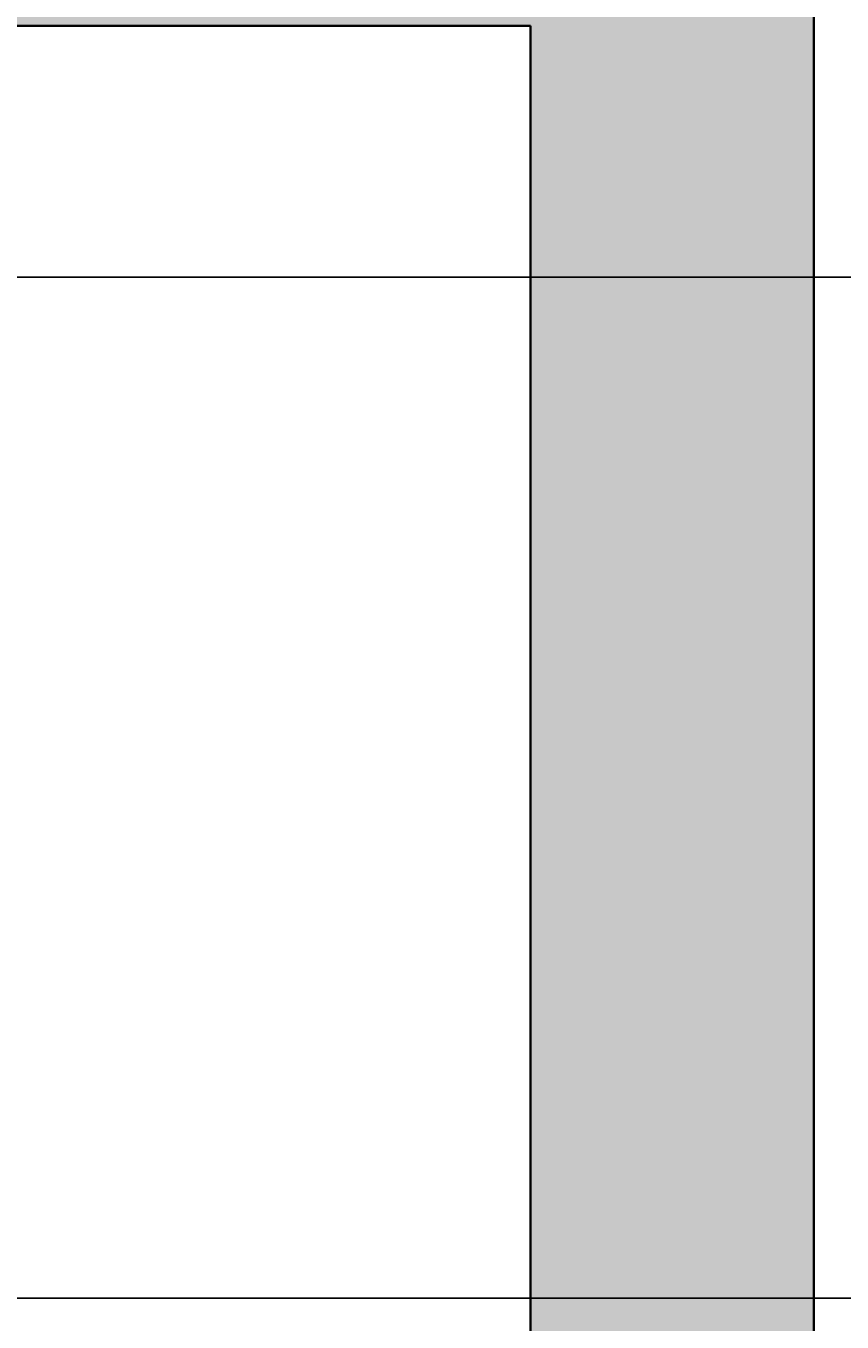
# Model space of a CAD drawing. Units: inches. Extents: x 1998 to 2588, y 1139 to 1977.
# Tile 120 of 134: x 2524 to 2550, y 1595 to 1637. Entities that reach past the tile are written whole.
import ezdxf

# ---------------------------------------------------------------- set-up
doc = ezdxf.new("R2010")
doc.units = ezdxf.units.IN
for name, color, linetype, lineweight in [('A-ANNO-DIMS', 2, 'Continuous', 18), ('A-WALL-PATT', 252, 'Continuous', 13), ('WALL', 200, 'Continuous', 35)]:
    doc.layers.add(name, color=color, linetype=linetype, lineweight=lineweight)
doc.styles.get("Standard").update_dxf_attribs({"font": 'arial.ttf'})
doc.dimstyles.get("Standard").update_dxf_attribs({"dimtxt": 0.18, "dimasz": 0.18, "dimexe": 0.18, "dimexo": 0.0625, "dimgap": 0.09, "dimtad": 0, "dimtih": 1, "dimtoh": 1, "dimdec": 4, "dimzin": 0, "dimdsep": 46, "dimtxsty": 'Standard', "dimcen": 0.09, "dimadec": 0, "dimazin": 0, "dimtfac": 1, "dimtdec": 4, "dimtofl": 0, "dimtmove": 0, "dimatfit": 3, "dimfxl": 1, "dimtolj": 1, "dimtzin": 0, "dimarcsym": 0})

# ---------------------------------------------------------------- blocks, each defined once
blk = doc.blocks.new('*D24')
at = {"layer": 'A-ANNO-DIMS', "color": 0, "lineweight": -2, "transparency": 16777216}
for p, q in [((2398.535, 1911.232), (2588.309, 1911.232)), ((2588.129, 1911.052), (2588.129, 1570.164)), ((2588.129, 1228.912), (2588.129, 1569.8)), ((2527.535, 1228.732), (2588.309, 1228.732))]:
    blk.add_line(p, q, dxfattribs=at)
at = {"layer": 'A-ANNO-DIMS', "color": 0, "transparency": 16777216}
for points in [[(2588.099, 1911.052), (2588.159, 1911.052), (2588.129, 1911.232)], [(2588.099, 1228.912), (2588.159, 1228.912), (2588.129, 1228.732)]]:
    blk.add_solid(points, dxfattribs=at)
at = {"layer": 'Defpoints', "color": 0, "transparency": 16777216}
for p in [(2398.473, 1911.232), (2588.129, 1911.232), (2527.473, 1228.732)]:
    blk.add_point(p, dxfattribs=at)
at = {"layer": 'A-ANNO-DIMS', "color": 0, "transparency": 16777216, "insert": (2588.129, 1569.982), "char_height": 0.18, "attachment_point": 5}
blk.add_mtext('\\A1;682.5', dxfattribs=at)
blk = doc.blocks.new('*D39')
at = {"layer": 'A-ANNO-DIMS', "color": 0, "lineweight": -2, "transparency": 16777216}
for p, q in [((2115.035, 1628.742), (2588.309, 1628.742)), ((2588.129, 1628.562), (2588.129, 1612.685)), ((2588.129, 1596.444), (2588.129, 1612.321)), ((2115.035, 1596.264), (2588.309, 1596.264))]:
    blk.add_line(p, q, dxfattribs=at)
at = {"layer": 'A-ANNO-DIMS', "color": 0, "transparency": 16777216}
for points in [[(2588.099, 1628.562), (2588.159, 1628.562), (2588.129, 1628.742)], [(2588.099, 1596.444), (2588.159, 1596.444), (2588.129, 1596.264)]]:
    blk.add_solid(points, dxfattribs=at)
at = {"layer": 'Defpoints', "color": 0, "transparency": 16777216}
for p in [(2114.973, 1628.742), (2588.129, 1628.742), (2114.973, 1596.264)]:
    blk.add_point(p, dxfattribs=at)
at = {"layer": 'A-ANNO-DIMS', "color": 0, "transparency": 16777216, "insert": (2588.129, 1612.503), "char_height": 0.18, "attachment_point": 5}
blk.add_mtext('\\A1;32.48', dxfattribs=at)

msp = doc.modelspace()

# ---------------------------------------------------------------- hatches: boundary and pattern name
at = {"layer": 'A-WALL-PATT'}
h = msp.add_hatch(color=256, dxfattribs=at)
h.dxf.hatch_style = 1
h.paths.add_polyline_path([(2527.4729, 1362.2324), (2510.9729, 1362.2324), (2510.9729, 1357.7324), (2518.4729, 1357.7324), (2518.4729, 1237.7324), (2503.1458, 1237.7324), (2503.1458, 1228.7324), (2527.4729, 1228.7324)])
h.paths.add_polyline_path([(2490.5682, 1362.2324), (2398.4729, 1362.2324), (2398.4729, 1357.7324), (2490.5682, 1357.7324)])
h.paths.add_polyline_path([(2224.9729, 1264.7324), (2222.9729, 1264.7324), (2222.9729, 1232.4125), (2341.4729, 1232.4125), (2341.4729, 1234.4125), (2224.9729, 1234.4125)])
h.paths.add_polyline_path([(2334.5332, 1273.7324), (2264.7638, 1273.7324), (2264.7638, 1269.5611, -0.043659), (2264.3413, 1264.7324), (2334.5332, 1264.7324)])
h.paths.add_polyline_path([(2236.9551, 1273.7324), (2234.4125, 1273.7324), (2234.4125, 1264.7324), (2236.9551, 1264.7324), (2236.9551, 1269.5611)])
h.paths.add_polyline_path([(2222.9729, 1293.2324), (2096.9729, 1293.2324), (2096.9729, 1345.0966), (2087.9729, 1345.0966), (2087.9729, 1284.2324), (2222.9729, 1284.2324), (2222.9729, 1285.137)])
h.paths.add_polyline_path([(2096.9729, 1458.7927), (2087.9729, 1458.7927), (2087.9729, 1417.7324), (2087.9729, 1413.2324), (2096.9729, 1413.2324), (2096.9729, 1417.7324)])
h.paths.add_polyline_path([(2096.9729, 1413.2324), (2087.9729, 1413.2324), (2087.9729, 1365.5012), (2096.9729, 1365.5012), (2096.9729, 1369.3358)])
h.paths.add_polyline_path([(2186.2943, 1417.7324), (2138.6074, 1417.7324), (2096.9729, 1417.7324), (2096.9729, 1413.2324), (2138.6074, 1413.2324), (2186.2943, 1413.2324)])
h.paths.add_polyline_path([(2181.4729, 1465.7324), (2176.9729, 1465.7324), (2176.9729, 1451.6434), (2181.4729, 1451.6434)])
h.paths.add_polyline_path([(2181.4729, 1422.1664), (2176.9729, 1422.1664), (2176.9729, 1417.7324), (2181.4729, 1417.7324)])
h.paths.add_polyline_path([(2063.9729, 1465.7324), (2087.9729, 1465.7324), (2087.9729, 1470.2324), (2059.4729, 1470.2324), (2059.4729, 1413.2324), (2087.9729, 1413.2324), (2087.9729, 1417.7324), (2063.9729, 1417.7324)])
h.paths.add_polyline_path([(2181.4729, 1755.2324), (2176.9729, 1755.2324), (2176.9729, 1748.6798), (2177.0513, 1748.6798), (2181.4729, 1748.6798)])
h.paths.add_polyline_path([(2227.4729, 1707.2324), (2220.4647, 1707.2324), (2220.4647, 1702.7324), (2222.9729, 1702.7324), (2222.9729, 1604.637), (2227.4729, 1604.637)])
h.paths.add_polyline_path([(2114.9729, 1702.7324), (2105.9729, 1702.7324), (2105.9729, 1628.4781, -0.0318759), (2110.1012, 1628.7416), (2114.9729, 1628.7416)])
h.paths.add_polyline_path([(2345.9729, 1739.3278), (2341.4729, 1739.3278), (2341.4729, 1647.5211), (2345.9729, 1647.5211)])
h.paths.add_polyline_path([(2350.6273, 1641.2324), (2345.9729, 1641.2324), (2345.9729, 1636.7324), (2350.6273, 1636.7324), (2350.6273, 1639.8729)])
h.paths.add_polyline_path([(2501.9729, 1641.2324), (2407.9729, 1641.2324), (2392.5005, 1641.2324), (2392.5005, 1639.8729), (2392.5005, 1636.7324), (2501.9729, 1636.7324)])
h.paths.add_polyline_path([(2510.9729, 1755.2324), (2501.9729, 1755.2324), (2501.9729, 1641.2324), (2510.9729, 1641.2324)])
h.paths.add_polyline_path([(2549.1786, 1641.2324), (2522.3775, 1641.2324), (2522.3775, 1636.7324), (2540.1786, 1636.7324), (2540.1786, 1480.7324), (2522.3775, 1480.7324), (2522.3775, 1476.2324), (2549.1786, 1476.2324)])
h.paths.add_polyline_path([(2498.1786, 1594.7324), (2407.9729, 1594.7324), (2407.9729, 1585.7324), (2416.9729, 1585.7324), (2489.1786, 1585.7324), (2489.1786, 1531.7324), (2416.9729, 1531.7324), (2407.9729, 1531.7324), (2407.9729, 1522.7324), (2498.1786, 1522.7324)])
h.paths.add_polyline_path([(2351.6437, 1480.7324), (2345.9729, 1480.7324), (2345.9729, 1476.2324), (2351.6437, 1476.2324), (2351.6437, 1477.5919)])
h.paths.add_polyline_path([(2501.9729, 1480.7324), (2498.1786, 1480.7324), (2407.9729, 1480.7324), (2393.5168, 1480.7324), (2393.5168, 1477.5919), (2393.5168, 1476.2324), (2501.9729, 1476.2324)])

# ---------------------------------------------------------------- linework, layer by layer
at = {"layer": 'WALL'}
for p, q in [((2549.1786, 1641.2324), (2549.1786, 1476.2324)), ((2540.1786, 1636.7324), (2522.3775, 1636.7324)), ((2522.3775, 1636.7324), (2540.1786, 1636.7324)), ((2540.1786, 1636.7324), (2540.1786, 1480.7324))]:
    msp.add_line(p, q, dxfattribs=at)

# ---------------------------------------------------------------- dimensions: what is measured, and where the dimension line sits
at = {"layer": 'A-ANNO-DIMS'}
for base, p1, p2, override, picture, middle in [((2588.1286, 1911.2324), (2527.4729, 1228.7324), (2398.4729, 1911.2324), {"dimdec": 1, "dimlfac": 1, "dimrnd": 0, "dimzin": 0, "dimdsep": 46, "dimlunit": 2}, '*D24', (2588.1286, 1569.9824)), ((2588.1286, 1628.7416), (2114.9729, 1596.2642), (2114.9729, 1628.7416), {"dimdec": 2, "dimlfac": 1, "dimrnd": 0, "dimzin": 0, "dimdsep": 46, "dimlunit": 2}, '*D39', (2588.1286, 1612.5029))]:
    dim = msp.add_linear_dim(base=base, p1=p1, p2=p2, angle=90, dimstyle='Standard', override=override, dxfattribs=at)
    dim.commit()
    dim.dimension.update_dxf_attribs({"geometry": picture, "text_midpoint": middle})

doc.saveas('drawing.dxf')
